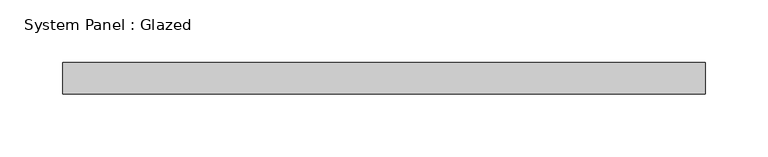
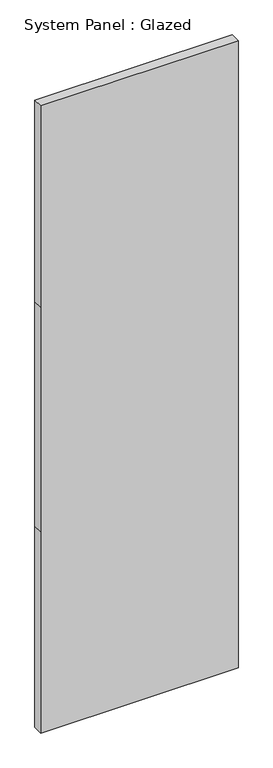
"""IFC4 building model written with IfcOpenShell, lengths in millimetres: plate geometry, System Panel : Glazed."""

from ifc_helpers import new_model, si_unit, frame, origin, place, context, project, spatial, polyline, outline, extrude, source, transform, mapped, element, save


def system_panel_glazed_f6e37d5f(model_context):
    return source(origin(), model_context, "Body", "SweptSolid", [
        extrude(outline(polyline([(0.0, -257.175), (0.0, 257.175), (554.5666667, 257.175), (1172.6333333, 257.175), (1727.2, 257.175), (1727.2, -257.175), (1172.6333333, -257.175), (554.5666667, -257.175), (0.0, -257.175)])), frame((0.0, 19.05, 0.0), z_axis=(0.0, 1.0, 0.0), x_axis=(0.0, 0.0, 1.0)), (0.0, 0.0, 1.0), 25.4),
    ])


if __name__ == "__main__":
    model = new_model("IFC4")
    model_context = context("Model", 3, world=origin())
    ifc_project = project(units=[si_unit("LENGTHUNIT", "METRE", prefix="MILLI")], contexts=[model_context])
    site = spatial("IfcSite", under=ifc_project)
    building = spatial("IfcBuilding", under=site)
    placement = place(None, origin())
    system_panel_glazed_shape = system_panel_glazed_f6e37d5f(model_context)
    element("IfcPlate", 1, ObjectType="System Panel : Glazed", at=placement, inside=building, context=model_context, shape_type="MappedRepresentation", body=[
        mapped(system_panel_glazed_shape, transform((0.0, 0.0, 0.0), x_axis=(1.0, 0.0, 0.0), y_axis=(0.0, 1.0, 0.0), z_axis=(0.0, 0.0, 1.0))),
    ])
    save(model, "model.ifc")

# Revit data of these elements
# Type "System Panel : Glazed"
#   Construction Type Id = "GSP4R"
#   Analytic Construction = "1/8 in Pilkington single glazing"
#   Visual Light Transmittance = 0.9
#   Solar Heat Gain Coefficient = 0.86
#   Heat Transfer Coefficient (U) = 1.18115 BTU/(h·ft²·°F)
#   Define Thermal Properties by = 1
# Element 1 (IfcPlate, "System Panel : Glazed")
#   Materials on its faces: "Glass"
# Materials
#   "Glass": class "Glass", colour RGB 0 128 192, transparency 0.75, Description = "Soda Lime Glass", Cost = 0
